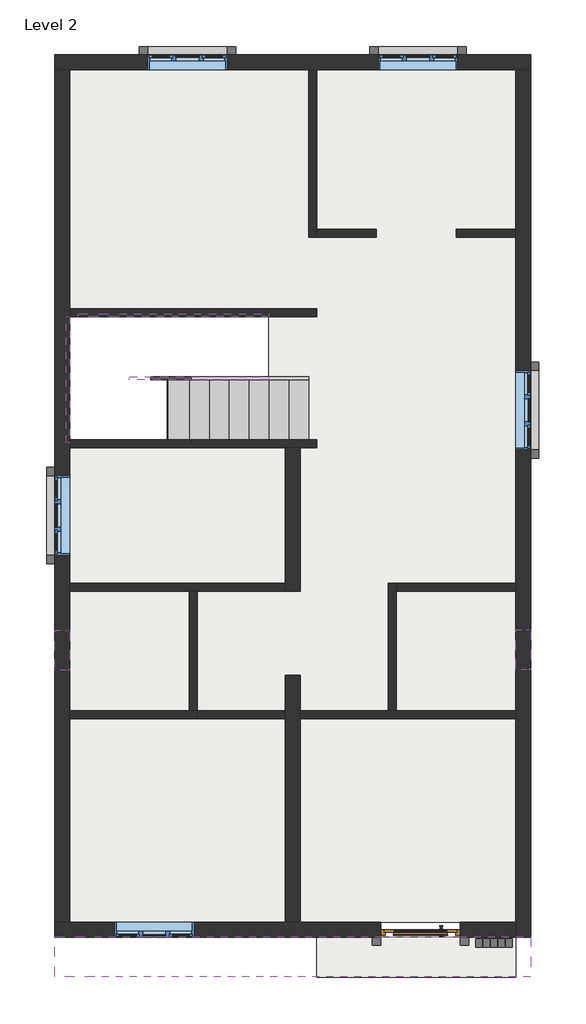
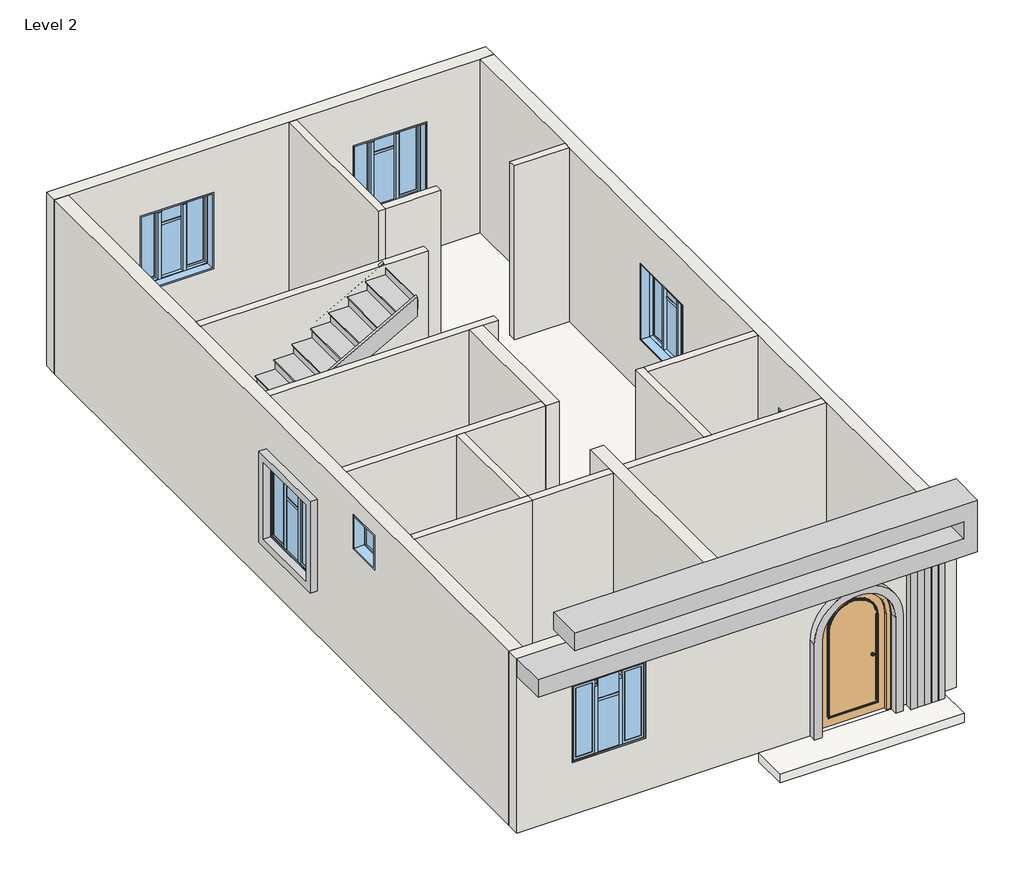
# One storey, incomplete: 18 walls, 7 proxies, 7 windows, 5 members, 4 slabs, 1 door, 1 stair flight.
"""IFC4 building model written with IfcOpenShell, lengths in millimetres."""

from ifc_helpers import new_model, si_unit, frame, origin, place, context, project, spatial, polyline, circle_curve, outline, extrude, faceted_brep, transform, mapped, element, save
from ifc_brep_helpers import plane_surface, revolved_surface, advanced_brep
from components import generic_models_13_generic_models_13_77cabad3, generic_models_14_generic_models_14_97bd1c4e, generic_models_20_generic_models_18_c69d9d0b, generic_models_3_generic_models_3_7bb868d1, generic_models_4_generic_models_4_8dd9e423, generic_models_5_generic_models_5_fe75d143, door_arched_single_french_glass_wood_exterior_1219_x_2134mm_7a906126, stair_flight_03b7873a, window_80340324, window_casement_triple_middle_transom_windows_4_x4_273a115f

model = new_model("IFC4")

# Units and contexts
model_context = context("Model", 3, world=origin())
ifc_project = project(units=[si_unit("LENGTHUNIT", "METRE", prefix="MILLI")], contexts=[model_context])

# Site, building, storey
site = spatial("IfcSite", under=ifc_project)
building = spatial("IfcBuilding", under=site)
storey = spatial("IfcBuildingStorey", under=building, Name="Level 2", Elevation=3352.8)

# Proxies
placement = place(None, origin())
generic_models_13_generic_models_13_shape = generic_models_13_generic_models_13_77cabad3(model_context)
element("IfcBuildingElementProxy", 1, Name="Generic Models 13 : Generic Models 13", ObjectType="Generic Models 13 : Generic Models 13", at=placement, inside=storey, context=model_context, shape_type="MappedRepresentation", body=[
    mapped(generic_models_13_generic_models_13_shape, transform((0.0, 0.0, 0.0), x_axis=(1.0, 0.0, 0.0), y_axis=(0.0, 1.0, 0.0), z_axis=(0.0, 0.0, 1.0))),
])
generic_models_14_generic_models_14_shape = generic_models_14_generic_models_14_97bd1c4e(model_context)
element("IfcBuildingElementProxy", 2, Name="Generic Models 14 : Generic Models 14", ObjectType="Generic Models 14 : Generic Models 14", at=placement, inside=storey, context=model_context, shape_type="MappedRepresentation", body=[
    mapped(generic_models_14_generic_models_14_shape, transform((0.0, 0.0, 0.0), x_axis=(1.0, 0.0, 0.0), y_axis=(0.0, 1.0, 0.0), z_axis=(0.0, 0.0, 1.0))),
])
element("IfcBuildingElementProxy", 3, Name="Generic Models 15 : Generic Models 14", ObjectType="Generic Models 15 : Generic Models 14", at=placement, inside=storey, context=model_context, shape_type="MappedRepresentation", body=[
    mapped(generic_models_14_generic_models_14_shape, transform((-3531.39375, 0.0, 0.0), x_axis=(1.0, 0.0, 0.0), y_axis=(0.0, 1.0, 0.0), z_axis=(0.0, 0.0, 1.0))),
])
generic_models_20_generic_models_18_shape = generic_models_20_generic_models_18_c69d9d0b(model_context)
element("IfcBuildingElementProxy", 4, Name="Generic Models 20 : Generic Models 18", ObjectType="Generic Models 20 : Generic Models 18", at=placement, inside=storey, context=model_context, shape_type="MappedRepresentation", body=[
    mapped(generic_models_20_generic_models_18_shape, transform((0.0, -4883.15, 3041.65), x_axis=(1.0, 0.0, 0.0), y_axis=(0.0, 1.0, 0.0), z_axis=(0.0, 0.0, 1.0))),
])
generic_models_3_generic_models_3_shape = generic_models_3_generic_models_3_7bb868d1(model_context)
element("IfcBuildingElementProxy", 5, Name="Generic Models 3 : Generic Models 3", ObjectType="Generic Models 3 : Generic Models 3", at=placement, inside=storey, context=model_context, shape_type="MappedRepresentation", body=[
    mapped(generic_models_3_generic_models_3_shape, transform((0.0, 0.0, 0.0), x_axis=(1.0, 0.0, 0.0), y_axis=(0.0, 1.0, 0.0), z_axis=(0.0, 0.0, 1.0))),
])
generic_models_4_generic_models_4_shape = generic_models_4_generic_models_4_8dd9e423(model_context)
element("IfcBuildingElementProxy", 6, Name="Generic Models 4 : Generic Models 4", ObjectType="Generic Models 4 : Generic Models 4", at=placement, inside=storey, context=model_context, shape_type="MappedRepresentation", body=[
    mapped(generic_models_4_generic_models_4_shape, transform((0.0, 0.0, 0.0), x_axis=(1.0, 0.0, 0.0), y_axis=(0.0, 1.0, 0.0), z_axis=(0.0, 0.0, 1.0))),
])
generic_models_5_generic_models_5_shape = generic_models_5_generic_models_5_fe75d143(model_context)
element("IfcBuildingElementProxy", 7, Name="Generic Models 5 : Generic Models 5", ObjectType="Generic Models 5 : Generic Models 5", at=placement, inside=storey, context=model_context, shape_type="MappedRepresentation", body=[
    mapped(generic_models_5_generic_models_5_shape, transform((0.0, 0.0, 0.0), x_axis=(1.0, 0.0, 0.0), y_axis=(0.0, 1.0, 0.0), z_axis=(0.0, 0.0, 1.0))),
])

# Door
door_arched_single_french_glass_wood_exterior_1219_x_2134mm_shape = door_arched_single_french_glass_wood_exterior_1219_x_2134mm_7a906126(model_context)
element("IfcDoor", 8, ObjectType="Door_Arched_Single_French_Glass_Wood_Exterior : 1219 x 2134mm", at=placement, inside=storey, context=model_context, shape_type="MappedRepresentation", body=[
    mapped(door_arched_single_french_glass_wood_exterior_1219_x_2134mm_shape, transform((-4097.4482439, -5608.2827462, 3352.8), x_axis=(-1.0, 0.0, 0.0), y_axis=(0.0, -1.0, 0.0), z_axis=(0.0, 0.0, 1.0))),
])

# Members
element("IfcMember", 9, ObjectType="Stringer - 2\" Width", at=placement, inside=storey, context=model_context, shape_type="SweptSolid", body=[
    extrude(outline(polyline([(3352.8, -5811.9482439), (3560.3983948, -5811.9482439), (5122.3333333, -8623.4311333), (5122.3333333, -9251.0527467), (3352.8, -6065.8927467), (3352.8, -5811.9482439)])), frame((0.0, 1846.6172538, 0.0), z_axis=(0.0, 1.0, 0.0), x_axis=(0.0, 0.0, 1.0)), (0.0, 0.0, 1.0), 50.8),
])
element("IfcMember", 10, ObjectType="Stringer - 2\" Width", at=placement, inside=storey, context=model_context, shape_type="SweptSolid", body=[
    extrude(outline(polyline([(-9471.1357439, 1846.6172538), (-9521.9357439, 1846.6172538), (-9521.9357439, 3777.0172538), (-9471.1357439, 3777.0172538), (-9471.1357439, 1846.6172538)])), frame((0.0, 0.0, 4817.5333333), z_axis=(0.0, 0.0, 1.0), x_axis=(1.0, 0.0, 0.0)), (0.0, 0.0, 1.0), 304.8),
])
element("IfcMember", 11, ObjectType="Stringer - 2\" Width", at=placement, inside=storey, context=model_context, shape_type="SweptSolid", body=[
    extrude(outline(polyline([(4817.5333333, -8712.6837411), (6090.3863873, -6421.5482439), (6439.0650614, -6421.5482439), (4817.5333333, -9340.3053545), (4817.5333333, -8712.6837411)])), frame((0.0, 3777.0172538, 0.0), z_axis=(0.0, 1.0, 0.0), x_axis=(0.0, 0.0, 1.0)), (0.0, 0.0, 1.0), 50.8),
])
element("IfcMember", 12, ObjectType="Stringer - 2\" Width", at=placement, inside=storey, context=model_context, shape_type="SweptSolid", body=[
    extrude(outline(polyline([(3352.8, -5811.9482439), (3560.3983948, -5811.9482439), (5056.1761726, -8504.3482439), (4707.4974984, -8504.3482439), (3352.8, -6065.8927467), (3352.8, -5811.9482439)])), frame((0.0, 2811.8172538, 0.0), z_axis=(0.0, 1.0, 0.0), x_axis=(0.0, 0.0, 1.0)), (0.0, 0.0, 1.0), 50.8),
])
element("IfcMember", 13, ObjectType="Stringer - 2\" Width", at=placement, inside=storey, context=model_context, shape_type="SweptSolid", body=[
    extrude(outline(polyline([(5253.7317281, -8555.1482439), (4905.053054, -8555.1482439), (6090.3863873, -6421.5482439), (6439.0650614, -6421.5482439), (5253.7317281, -8555.1482439)])), frame((0.0, 2811.8172538, 0.0), z_axis=(0.0, 1.0, 0.0), x_axis=(0.0, 0.0, 1.0)), (0.0, 0.0, 1.0), 50.8),
])

# Slabs
element("IfcSlab", 14, ObjectType="6\" flooring bathroom second lvl", at=placement, inside=storey, context=model_context, shape_type="SweptSolid", body=[
    extrude(outline(polyline([(-7640.7482439, -426.6827462), (-7640.7482439, -2255.4827462), (-9471.1357439, -2255.4827462), (-9471.1357439, -426.6827462), (-7640.7482439, -426.6827462)])), frame((0.0, 0.0, 3200.4), z_axis=(0.0, 0.0, 1.0), x_axis=(1.0, 0.0, 0.0)), (0.0, 0.0, 1.0), 152.4),
    extrude(outline(polyline([(-2636.9482439, -426.6827462), (-2636.9482439, -2255.4827462), (-4465.7482439, -2255.4827462), (-4465.7482439, -426.6827462), (-2636.9482439, -426.6827462)])), frame((0.0, 0.0, 3200.4), z_axis=(0.0, 0.0, 1.0), x_axis=(1.0, 0.0, 0.0)), (0.0, 0.0, 1.0), 152.4),
])
element("IfcSlab", 15, ObjectType="6\" flooring bathroom second lvl", at=placement, inside=storey, context=model_context, shape_type="SweptSolid", body=[
    extrude(outline(polyline([(-2635.3607439, -5722.5827462), (-2635.3607439, -6341.8842658), (-5683.3607439, -6341.8842658), (-5683.3607439, -5722.5827462), (-2635.3607439, -5722.5827462)])), frame((0.0, 0.0, 3200.4), z_axis=(0.0, 0.0, 1.0), x_axis=(1.0, 0.0, 0.0)), (0.0, 0.0, 1.0), 152.4),
])
element("IfcSlab", 16, ObjectType="flooring 6\"", at=placement, inside=storey, context=model_context, shape_type="SweptSolid", body=[
    extrude(outline(polyline([(-9471.1357439, 3904.0172538), (-9471.1357439, 7563.2047538), (-5811.9482439, 7563.2047538), (-5811.9482439, 4996.2172538), (-4770.5482439, 4996.2172538), (-4770.5482439, 5123.2172538), (-5684.9482439, 5123.2172538), (-5684.9482439, 7563.2047538), (-2636.9482439, 7563.2047538), (-2636.9482439, 5123.2172538), (-3551.3482439, 5123.2172538), (-3551.3482439, 4996.2172538), (-2636.9482439, 4996.2172538), (-2636.9482439, -299.6827462), (-4592.7482439, -299.6827462), (-4592.7482439, -2255.4827462), (-5936.4082439, -2255.4827462), (-5936.4082439, -1709.3827462), (-6165.0082439, -1709.3827462), (-6165.0082439, -2255.4827462), (-6170.0882439, -2255.4827462), (-7513.7482439, -2255.4827462), (-7513.7482439, -426.6827462), (-5936.4082439, -426.6827462), (-5936.4082439, 1770.4172538), (-5684.9482439, 1770.4172538), (-5684.9482439, 1897.4172538), (-5811.9482439, 1897.4172538), (-5811.9482439, 2862.6172538), (-6421.5482439, 2862.6172538), (-6421.5482439, 3777.0172538), (-5684.9482439, 3777.0172538), (-5684.9482439, 3904.0172538), (-9471.1357439, 3904.0172538)])), frame((0.0, 0.0, 3200.4), z_axis=(0.0, 0.0, 1.0), x_axis=(1.0, 0.0, 0.0)), (0.0, 0.0, 1.0), 152.4),
])
element("IfcSlab", 17, ObjectType="flooring 6\"", at=placement, inside=storey, context=model_context, shape_type="SweptSolid", body=[
    extrude(outline(polyline([(-6165.0082439, 1770.4172538), (-6165.0082439, -299.6827462), (-9471.1357439, -299.6827462), (-9471.1357439, 1770.4172538), (-6165.0082439, 1770.4172538)])), frame((0.0, 0.0, 3327.4), z_axis=(0.0, 0.0, 1.0), x_axis=(1.0, 0.0, 0.0)), (0.0, 0.0, 1.0), 152.4),
    extrude(outline(polyline([(-6170.0882439, -5493.9827462), (-9471.1357439, -5493.9827462), (-9471.1357439, -2382.4827462), (-6170.0882439, -2382.4827462), (-6170.0882439, -5493.9827462)])), frame((0.0, 0.0, 3327.4), z_axis=(0.0, 0.0, 1.0), x_axis=(1.0, 0.0, 0.0)), (0.0, 0.0, 1.0), 152.4),
    extrude(outline(polyline([(-2636.9482439, -2382.4827462), (-2636.9482439, -5493.9827462), (-5936.4082439, -5493.9827462), (-5936.4082439, -2382.4827462), (-2636.9482439, -2382.4827462)])), frame((0.0, 0.0, 3327.4), z_axis=(0.0, 0.0, 1.0), x_axis=(1.0, 0.0, 0.0)), (0.0, 0.0, 1.0), 152.4),
])

# Stair flight
stair_flight_shape = stair_flight_03b7873a(model_context)
element("IfcStairFlight", 18, ObjectType="2\" Tread 1\" Nosing 1/4\" Riser", at=placement, inside=storey, context=model_context, shape_type="MappedRepresentation", body=[
    mapped(stair_flight_shape, transform((0.0, 0.0, 0.0), x_axis=(1.0, 0.0, 0.0), y_axis=(0.0, 1.0, 0.0), z_axis=(0.0, 0.0, 1.0))),
])

# Walls
element("IfcWall", 19, ObjectType="INNER WALL 5\"", at=placement, inside=storey, context=model_context, shape_type="SweptSolid", body=[
    extrude(outline(polyline([(-5684.9482439, 3777.0172538), (-9471.1357439, 3777.0172538), (-9471.1357439, 3904.0172538), (-5684.9482439, 3904.0172538), (-5684.9482439, 3777.0172538)])), frame((0.0, 0.0, 3352.8), z_axis=(0.0, 0.0, 1.0), x_axis=(1.0, 0.0, 0.0)), (0.0, 0.0, 1.0), 3048.0),
])
element("IfcWall", 20, ObjectType="INNER WALL 5\"", at=placement, inside=storey, context=model_context, shape_type="Brep", body=[
    faceted_brep([(-9471.1357439, 1770.4172538, 3352.8), (-6165.0082439, 1770.4172538, 3352.8), (-5936.4082439, 1770.4172538, 3352.8), (-5684.9482439, 1770.4172538, 3352.8), (-5684.9482439, 1770.4172538, 6400.8), (-5936.4082439, 1770.4172538, 6400.8), (-6165.0082439, 1770.4172538, 6400.8), (-9471.1357439, 1770.4172538, 6400.8), (-9471.1357439, 1897.4172538, 3352.8), (-9471.1357439, 1897.4172538, 6400.8), (-5684.9482439, 1897.4172538, 6400.8), (-5684.9482439, 1897.4172538, 3352.8)], [[[0, 1, 2, 3, 4, 5, 6, 7]], [[8, 9, 10, 11]], [[3, 2, 1, 0, 8, 11]], [[4, 3, 11, 10]], [[7, 6, 5, 4, 10, 9]], [[0, 7, 9, 8]]]),
])
element("IfcWall", 21, ObjectType="INNER WALL 5\"", at=placement, inside=storey, context=model_context, shape_type="Brep", body=[
    faceted_brep([(-9471.1357439, -426.6827462, 3352.8), (-7640.7482439, -426.6827462, 3352.8), (-7513.7482439, -426.6827462, 3352.8), (-6165.0082439, -426.6827462, 3352.8), (-6165.0082439, -426.6827462, 6400.8), (-7513.7482439, -426.6827462, 6400.8), (-7640.7482439, -426.6827462, 6400.8), (-9471.1357439, -426.6827462, 6400.8), (-9471.1357439, -299.6827462, 3352.8), (-9471.1357439, -299.6827462, 6400.8), (-6165.0082439, -299.6827462, 6400.8), (-6165.0082439, -299.6827462, 3352.8)], [[[0, 1, 2, 3, 4, 5, 6, 7]], [[8, 9, 10, 11]], [[3, 2, 1, 0, 8, 11]], [[7, 6, 5, 4, 10, 9]], [[4, 3, 11, 10]], [[0, 7, 9, 8]]]),
])
element("IfcWall", 22, ObjectType="INNER WALL 5\"", at=placement, inside=storey, context=model_context, shape_type="Brep", body=[
    faceted_brep([(-9469.5482439, -2382.4827462, 3352.8), (-7513.7482439, -2382.4827462, 3352.8), (-7513.7482439, -2382.4827462, 6400.8), (-9469.5482439, -2382.4827462, 6400.8), (-9469.5482439, -2255.4827462, 3352.8), (-9469.5482439, -2255.4827462, 6400.8), (-7640.7482439, -2255.4827462, 6400.8), (-7513.7482439, -2255.4827462, 6400.8), (-7513.7482439, -2255.4827462, 3352.8), (-7640.7482439, -2255.4827462, 3352.8)], [[[0, 1, 2, 3]], [[4, 5, 6, 7, 8, 9]], [[1, 0, 4, 9, 8]], [[3, 2, 7, 6, 5]], [[0, 3, 5, 4]], [[2, 1, 8, 7]]]),
])
element("IfcWall", 23, ObjectType="INNER WALL 5\"", at=placement, inside=storey, context=model_context, shape_type="SweptSolid", body=[
    extrude(outline(polyline([(-7513.7482439, -426.6827462), (-7513.7482439, -2255.4827462), (-7640.7482439, -2255.4827462), (-7640.7482439, -426.6827462), (-7513.7482439, -426.6827462)])), frame((0.0, 0.0, 3352.8), z_axis=(0.0, 0.0, 1.0), x_axis=(1.0, 0.0, 0.0)), (0.0, 0.0, 1.0), 3048.0),
])
element("IfcWall", 24, ObjectType="INNER WALL 5\"", at=placement, inside=storey, context=model_context, shape_type="SweptSolid", body=[
    extrude(outline(polyline([(-7513.7482439, -2255.4827462), (-6170.0882439, -2255.4827462), (-6170.0882439, -2382.4827462), (-7513.7482439, -2382.4827462), (-7513.7482439, -2255.4827462)])), frame((0.0, 0.0, 3352.8), z_axis=(0.0, 0.0, 1.0), x_axis=(1.0, 0.0, 0.0)), (0.0, 0.0, 1.0), 3048.0),
])
element("IfcWall", 25, ObjectType="INNER WALL 5\"", at=placement, inside=storey, context=model_context, shape_type="Brep", body=[
    faceted_brep([(-5936.4082439, -2382.4827462, 3352.8), (-2636.9482439, -2382.4827462, 3352.8), (-2636.9482439, -2382.4827462, 6400.8), (-5936.4082439, -2382.4827462, 6400.8), (-5936.4082439, -2255.4827462, 3352.8), (-5936.4082439, -2255.4827462, 6400.8), (-4592.7482439, -2255.4827462, 6400.8), (-4465.7482439, -2255.4827462, 6400.8), (-2636.9482439, -2255.4827462, 6400.8), (-2636.9482439, -2255.4827462, 3352.8), (-4465.7482439, -2255.4827462, 3352.8), (-4592.7482439, -2255.4827462, 3352.8)], [[[0, 1, 2, 3]], [[4, 5, 6, 7, 8, 9, 10, 11]], [[1, 0, 4, 11, 10, 9]], [[3, 2, 8, 7, 6, 5]], [[0, 3, 5, 4]], [[2, 1, 9, 8]]]),
])
element("IfcWall", 26, ObjectType="INNER WALL 5\"", at=placement, inside=storey, context=model_context, shape_type="Brep", body=[
    faceted_brep([(-4465.7482439, -2255.4827462, 3352.8), (-4465.7482439, -426.6827462, 3352.8), (-4465.7482439, -299.6827462, 3352.8), (-4465.7482439, -299.6827462, 6400.8), (-4465.7482439, -426.6827462, 6400.8), (-4465.7482439, -2255.4827462, 6400.8), (-4592.7482439, -2255.4827462, 3352.8), (-4592.7482439, -2255.4827462, 6400.8), (-4592.7482439, -299.6827462, 6400.8), (-4592.7482439, -299.6827462, 3352.8)], [[[0, 1, 2, 3, 4, 5]], [[6, 7, 8, 9]], [[2, 1, 0, 6, 9]], [[5, 4, 3, 8, 7]], [[0, 5, 7, 6]], [[3, 2, 9, 8]]]),
])
element("IfcWall", 27, ObjectType="INNER WALL 5\"", at=placement, inside=storey, context=model_context, shape_type="SweptSolid", body=[
    extrude(outline(polyline([(-2636.9482439, -426.6827462), (-4465.7482439, -426.6827462), (-4465.7482439, -299.6827462), (-2636.9482439, -299.6827462), (-2636.9482439, -426.6827462)])), frame((0.0, 0.0, 3352.8), z_axis=(0.0, 0.0, 1.0), x_axis=(1.0, 0.0, 0.0)), (0.0, 0.0, 1.0), 3048.0),
])
element("IfcWall", 28, ObjectType="INNER WALL 5\"", at=placement, inside=storey, context=model_context, shape_type="Brep", body=[
    faceted_brep([(-5811.9482439, 7563.2047538, 3352.8), (-5811.9482439, 4996.2172538, 3352.8), (-5811.9482439, 4996.2172538, 6400.8), (-5811.9482439, 7563.2047538, 6400.8), (-5684.9482439, 7563.2047538, 3352.8), (-5684.9482439, 7563.2047538, 6400.8), (-5684.9482439, 5123.2172538, 6400.8), (-5684.9482439, 4996.2172538, 6400.8), (-5684.9482439, 4996.2172538, 3352.8), (-5684.9482439, 5123.2172538, 3352.8)], [[[0, 1, 2, 3]], [[4, 5, 6, 7, 8, 9]], [[1, 0, 4, 9, 8]], [[3, 2, 7, 6, 5]], [[0, 3, 5, 4]], [[2, 1, 8, 7]]]),
])
element("IfcWall", 29, ObjectType="INNER WALL 5\"", at=placement, inside=storey, context=model_context, shape_type="SweptSolid", body=[
    extrude(outline(polyline([(-4770.5482439, 4996.2172538), (-5684.9482439, 4996.2172538), (-5684.9482439, 5123.2172538), (-4770.5482439, 5123.2172538), (-4770.5482439, 4996.2172538)])), frame((0.0, 0.0, 3352.8), z_axis=(0.0, 0.0, 1.0), x_axis=(1.0, 0.0, 0.0)), (0.0, 0.0, 1.0), 3048.0),
])
element("IfcWall", 30, ObjectType="INNER WALL 5\"", at=placement, inside=storey, context=model_context, shape_type="SweptSolid", body=[
    extrude(outline(polyline([(-2636.9482439, 4996.2172538), (-3551.3482439, 4996.2172538), (-3551.3482439, 5123.2172538), (-2636.9482439, 5123.2172538), (-2636.9482439, 4996.2172538)])), frame((0.0, 0.0, 3352.8), z_axis=(0.0, 0.0, 1.0), x_axis=(1.0, 0.0, 0.0)), (0.0, 0.0, 1.0), 3048.0),
])
element("IfcWall", 31, ObjectType="WALL 9\"", at=placement, inside=storey, context=model_context, shape_type="Brep", body=[
    faceted_brep([(-9699.7357439, 7563.2047538, 3352.8), (-9471.1357439, 7563.2047538, 3352.8), (-5811.9482439, 7563.2047538, 3352.8), (-5684.9482439, 7563.2047538, 3352.8), (-2636.9482439, 7563.2047538, 3352.8), (-2408.3482439, 7563.2047538, 3352.8), (-2408.3482439, 7563.2047538, 6400.8), (-2636.9482439, 7563.2047538, 6400.8), (-5684.9482439, 7563.2047538, 6400.8), (-5811.9482439, 7563.2047538, 6400.8), (-9471.1357439, 7563.2047538, 6400.8), (-9699.7357439, 7563.2047538, 6400.8), (-3525.9482439, 7563.2047538, 5613.4), (-3525.9482439, 7563.2047538, 4267.2), (-4745.1482439, 7563.2047538, 4267.2), (-4745.1482439, 7563.2047538, 5613.4), (-7057.3419939, 7563.2047538, 5613.4), (-7057.3419939, 7563.2047538, 4267.2), (-8276.5419939, 7563.2047538, 4267.2), (-8276.5419939, 7563.2047538, 5613.4), (-9699.7357439, 7791.8047538, 3352.8), (-9699.7357439, 7791.8047538, 6400.8), (-2408.3482439, 7791.8047538, 6400.8), (-2408.3482439, 7791.8047538, 3352.8), (-3525.9482439, 7791.8047538, 5613.4), (-4745.1482439, 7791.8047538, 5613.4), (-4745.1482439, 7791.8047538, 4267.2), (-3525.9482439, 7791.8047538, 4267.2), (-7057.3419939, 7791.8047538, 5613.4), (-8276.5419939, 7791.8047538, 5613.4), (-8276.5419939, 7791.8047538, 4267.2), (-7057.3419939, 7791.8047538, 4267.2)], [[[0, 1, 2, 3, 4, 5, 6, 7, 8, 9, 10, 11], [12, 13, 14, 15], [16, 17, 18, 19]], [[20, 21, 22, 23], [24, 25, 26, 27], [28, 29, 30, 31]], [[5, 4, 3, 2, 1, 0, 20, 23]], [[11, 10, 9, 8, 7, 6, 22, 21]], [[6, 5, 23, 22]], [[0, 11, 21, 20]], [[13, 12, 24, 27]], [[14, 13, 27, 26]], [[15, 14, 26, 25]], [[12, 15, 25, 24]], [[17, 16, 28, 31]], [[18, 17, 31, 30]], [[19, 18, 30, 29]], [[16, 19, 29, 28]]]),
])
element("IfcWall", 32, ObjectType="WALL 9\"", at=placement, inside=storey, context=model_context, shape_type="Brep", body=[
    faceted_brep([(-2636.9482439, 7563.2047538, 3352.8), (-2636.9482439, 5123.2172538, 3352.8), (-2636.9482439, 4996.2172538, 3352.8), (-2636.9482439, -299.6827462, 3352.8), (-2636.9482439, -426.6827462, 3352.8), (-2636.9482439, -2255.4827462, 3352.8), (-2636.9482439, -2382.4827462, 3352.8), (-2636.9482439, -5493.9827462, 3352.8), (-2636.9482439, -5722.5827462, 3352.8), (-2636.9482439, -5722.5827462, 6400.8), (-2636.9482439, -5493.9827462, 6400.8), (-2636.9482439, -2382.4827462, 6400.8), (-2636.9482439, -2255.4827462, 6400.8), (-2636.9482439, -426.6827462, 6400.8), (-2636.9482439, -299.6827462, 6400.8), (-2636.9482439, 4996.2172538, 6400.8), (-2636.9482439, 5123.2172538, 6400.8), (-2636.9482439, 7563.2047538, 6400.8), (-2636.9482439, 1738.6672538, 5613.4), (-2636.9482439, 1738.6672538, 4267.2), (-2636.9482439, 2957.8672538, 4267.2), (-2636.9482439, 2957.8672538, 5613.4), (-2636.9482439, -1626.8327462, 5486.4), (-2636.9482439, -1626.8327462, 4876.8), (-2636.9482439, -1017.2327462, 4876.8), (-2636.9482439, -1017.2327462, 5486.4), (-2408.3482439, 7563.2047538, 3352.8), (-2408.3482439, 7563.2047538, 6400.8), (-2408.3482439, -5722.5827462, 6400.8), (-2408.3482439, -5722.5827462, 3352.8), (-2408.3482439, 1738.6672538, 5613.4), (-2408.3482439, 2957.8672538, 5613.4), (-2408.3482439, 2957.8672538, 4267.2), (-2408.3482439, 1738.6672538, 4267.2), (-2408.3482439, -1626.8327462, 5486.4), (-2408.3482439, -1017.2327462, 5486.4), (-2408.3482439, -1017.2327462, 4876.8), (-2408.3482439, -1626.8327462, 4876.8)], [[[0, 1, 2, 3, 4, 5, 6, 7, 8, 9, 10, 11, 12, 13, 14, 15, 16, 17], [18, 19, 20, 21], [22, 23, 24, 25]], [[26, 27, 28, 29], [30, 31, 32, 33], [34, 35, 36, 37]], [[8, 7, 6, 5, 4, 3, 2, 1, 0, 26, 29]], [[17, 16, 15, 14, 13, 12, 11, 10, 9, 28, 27]], [[0, 17, 27, 26]], [[9, 8, 29, 28]], [[19, 18, 30, 33]], [[20, 19, 33, 32]], [[21, 20, 32, 31]], [[18, 21, 31, 30]], [[23, 22, 34, 37]], [[24, 23, 37, 36]], [[25, 24, 36, 35]], [[22, 25, 35, 34]]]),
])
element("IfcWall", 33, ObjectType="WALL 9\"", at=placement, inside=storey, context=model_context, shape_type="AdvancedBrep", body=[
    advanced_brep(
    [(-4707.0482439, -5493.9827462, 5031.4), (-4707.0482439, -5493.9827462, 3352.8), (-5936.4082439, -5493.9827462, 3352.8), (-6165.0082439, -5493.9827462, 3352.8), (-9471.1357439, -5493.9827462, 3352.8), (-9699.7357439, -5493.9827462, 3352.8), (-9699.7357439, -5493.9827462, 6400.8), (-9471.1357439, -5493.9827462, 6400.8), (-6165.0082439, -5493.9827462, 6400.8), (-5936.4082439, -5493.9827462, 6400.8), (-2636.9482439, -5493.9827462, 6400.8), (-2636.9482439, -5493.9827462, 3352.8), (-3487.8482439, -5493.9827462, 3352.8), (-3487.8482439, -5493.9827462, 5031.4), (-8783.2719939, -5493.9827462, 5613.4), (-8783.2719939, -5493.9827462, 4267.2), (-7564.0719939, -5493.9827462, 4267.2), (-7564.0719939, -5493.9827462, 5613.4), (-9699.7357439, -5722.5827462, 3352.8), (-4707.0482439, -5722.5827462, 3352.8), (-4707.0482439, -5722.5827462, 5031.4), (-3487.8482439, -5722.5827462, 5031.4), (-3487.8482439, -5722.5827462, 3352.8), (-2636.9482439, -5722.5827462, 3352.8), (-2636.9482439, -5722.5827462, 6400.8), (-9699.7357439, -5722.5827462, 6400.8), (-8783.2719939, -5722.5827462, 5613.4), (-7564.0719939, -5722.5827462, 5613.4), (-7564.0719939, -5722.5827462, 4267.2), (-8783.2719939, -5722.5827462, 4267.2)],
    [
        (0, 1),
        (1, 2),
        (2, 3),
        (3, 4),
        (4, 5),
        (5, 6),
        (6, 7),
        (7, 8),
        (8, 9),
        (9, 10),
        (10, 11),
        (11, 12),
        (12, 13),
        (13, 0, circle_curve(frame((-4097.4482439, -5493.9827462, 5031.4), z_axis=(0.0, -1.0, 0.0), x_axis=(-1.0, 0.0, 0.0)), 609.6)),
        (14, 15),
        (15, 16),
        (16, 17),
        (17, 14),
        (18, 19),
        (19, 20),
        (20, 21, circle_curve(frame((-4097.4482439, -5722.5827462, 5031.4), z_axis=(0.0, 1.0, 0.0), x_axis=(-1.0, 0.0, 0.0)), 609.6)),
        (21, 22),
        (22, 23),
        (23, 24),
        (24, 25),
        (25, 18),
        (26, 27),
        (27, 28),
        (28, 29),
        (29, 26),
        (11, 23),
        (22, 12),
        (1, 19),
        (18, 5),
        (6, 25),
        (24, 10),
        (14, 26),
        (29, 15),
        (28, 16),
        (27, 17),
        (20, 0),
        (13, 21),
    ],
    [
        plane_surface(frame((-2408.3482439, -5493.9827462, 3352.8), z_axis=(0.0, 1.0, 0.0), x_axis=(-1.0, 0.0, 0.0))),
        plane_surface(frame((-2408.3482439, -5722.5827462, 3352.8), z_axis=(0.0, -1.0, 0.0), x_axis=(1.0, 0.0, 0.0))),
        plane_surface(frame((-2522.6482439, -5493.9827462, 3352.8), z_axis=(0.0, 0.0, -1.0), x_axis=(0.0, -1.0, 0.0))),
        plane_surface(frame((-9585.4357439, -5493.9827462, 6400.8), z_axis=(0.0, 0.0, 1.0), x_axis=(0.0, -1.0, 0.0))),
        plane_surface(frame((-2636.9482439, 7551.109711, 3352.8), z_axis=(1.0, 0.0, 0.0), x_axis=(0.0, -1.0, 0.0))),
        plane_surface(frame((-9699.7357439, -5722.5827462, 3352.8), z_axis=(-1.0, 0.0, 0.0), x_axis=(0.0, -1.0, 0.0))),
        plane_surface(frame((-8783.2719939, -5493.9827462, 5613.4), z_axis=(1.0, 0.0, 0.0), x_axis=(0.0, -1.0, 0.0))),
        plane_surface(frame((-8783.2719939, -5493.9827462, 4267.2), z_axis=(0.0, 0.0, 1.0), x_axis=(0.0, -1.0, 0.0))),
        plane_surface(frame((-7564.0719939, -5493.9827462, 4267.2), z_axis=(-1.0, 0.0, 0.0), x_axis=(0.0, -1.0, 0.0))),
        plane_surface(frame((-7564.0719939, -5493.9827462, 5613.4), z_axis=(0.0, 0.0, -1.0), x_axis=(0.0, -1.0, 0.0))),
        revolved_surface(polyline([(-4707.048243900001, -5493.9827462, 5031.4), (-4707.048243900001, -5722.5827462, 5031.4)]), (-4097.4482439, -5493.9827462, 5031.4), (0.0, 1.0, 0.0)),
        plane_surface(frame((-3487.8482439, -5722.5827462, 5031.4), z_axis=(-1.0, 0.0, 0.0), x_axis=(0.0, 1.0, 0.0))),
        plane_surface(frame((-4707.0482439, -5722.5827462, 3352.8), z_axis=(1.0, 0.0, 0.0), x_axis=(0.0, 1.0, 0.0))),
    ],
    [
        (0, [[1, 2, 3, 4, 5, 6, 7, 8, 9, 10, 11, 12, 13, 14], [15, 16, 17, 18]]),
        (1, [[19, 20, 21, 22, 23, 24, 25, 26], [27, 28, 29, 30]]),
        (2, [[-12, 31, -23, 32]]),
        (2, [[-5, -4, -3, -2, 33, -19, 34]]),
        (3, [[-10, -9, -8, -7, 35, -25, 36]]),
        (4, [[-11, -36, -24, -31]]),
        (5, [[-6, -34, -26, -35]]),
        (6, [[-15, 37, -30, 38]]),
        (7, [[-16, -38, -29, 39]]),
        (8, [[-17, -39, -28, 40]]),
        (9, [[-18, -40, -27, -37]]),
        (10, [[-21, 41, -14, 42]]),
        (11, [[-22, -42, -13, -32]]),
        (12, [[-20, -33, -1, -41]]),
    ],
),
])
element("IfcWall", 34, ObjectType="WALL 9\"", at=placement, inside=storey, context=model_context, shape_type="Brep", body=[
    faceted_brep([(-9471.1357439, -5493.9827462, 3352.8), (-9471.1357439, -426.6827462, 3352.8), (-9471.1357439, -299.6827462, 3352.8), (-9471.1357439, 1770.4172538, 3352.8), (-9471.1357439, 1897.4172538, 3352.8), (-9471.1357439, 3777.0172538, 3352.8), (-9471.1357439, 3904.0172538, 3352.8), (-9471.1357439, 7563.2047538, 3352.8), (-9471.1357439, 7563.2047538, 6400.8), (-9471.1357439, 3904.0172538, 6400.8), (-9471.1357439, 3777.0172538, 6400.8), (-9471.1357439, 1897.4172538, 6400.8), (-9471.1357439, 1770.4172538, 6400.8), (-9471.1357439, -299.6827462, 6400.8), (-9471.1357439, -426.6827462, 6400.8), (-9471.1357439, -5493.9827462, 6400.8), (-9471.1357439, 1344.9672538, 5613.4), (-9471.1357439, 1344.9672538, 4267.2), (-9471.1357439, 125.7672538, 4267.2), (-9471.1357439, 125.7672538, 5613.4), (-9471.1357439, -1633.1827462, 6096.0), (-9471.1357439, -1023.5827462, 6096.0), (-9471.1357439, -1023.5827462, 5486.4), (-9471.1357439, -1633.1827462, 5486.4), (-9699.7357439, -5493.9827462, 3352.8), (-9699.7357439, -5493.9827462, 6400.8), (-9699.7357439, 7563.2047538, 6400.8), (-9699.7357439, 7563.2047538, 3352.8), (-9699.7357439, 1344.9672538, 5613.4), (-9699.7357439, 125.7672538, 5613.4), (-9699.7357439, 125.7672538, 4267.2), (-9699.7357439, 1344.9672538, 4267.2), (-9699.7357439, -1633.1827462, 6096.0), (-9699.7357439, -1633.1827462, 5486.4), (-9699.7357439, -1023.5827462, 5486.4), (-9699.7357439, -1023.5827462, 6096.0)], [[[0, 1, 2, 3, 4, 5, 6, 7, 8, 9, 10, 11, 12, 13, 14, 15], [16, 17, 18, 19], [20, 21, 22, 23]], [[24, 25, 26, 27], [28, 29, 30, 31], [32, 33, 34, 35]], [[7, 6, 5, 4, 3, 2, 1, 0, 24, 27]], [[15, 14, 13, 12, 11, 10, 9, 8, 26, 25]], [[0, 15, 25, 24]], [[8, 7, 27, 26]], [[17, 16, 28, 31]], [[18, 17, 31, 30]], [[19, 18, 30, 29]], [[16, 19, 29, 28]], [[33, 32, 20, 23]], [[34, 33, 23, 22]], [[35, 34, 22, 21]], [[32, 35, 21, 20]]]),
])
element("IfcWall", 35, ObjectType="WALL 9\"", at=placement, inside=storey, context=model_context, shape_type="Brep", body=[
    faceted_brep([(-5936.4082439, -5493.9827462, 3352.8), (-5936.4082439, -2382.4827462, 3352.8), (-5936.4082439, -2255.4827462, 3352.8), (-5936.4082439, -1709.3827462, 3352.8), (-5936.4082439, -1709.3827462, 6400.8), (-5936.4082439, -2255.4827462, 6400.8), (-5936.4082439, -2382.4827462, 6400.8), (-5936.4082439, -5493.9827462, 6400.8), (-6165.0082439, -5493.9827462, 3352.8), (-6165.0082439, -5493.9827462, 6400.8), (-6165.0082439, -1709.3827462, 6400.8), (-6165.0082439, -1709.3827462, 3352.8)], [[[0, 1, 2, 3, 4, 5, 6, 7]], [[8, 9, 10, 11]], [[3, 2, 1, 0, 8, 11]], [[4, 3, 11, 10]], [[7, 6, 5, 4, 10, 9]], [[0, 7, 9, 8]]]),
])
element("IfcWall", 36, ObjectType="WALL 9\"", at=placement, inside=storey, context=model_context, shape_type="Brep", body=[
    faceted_brep([(-6165.0082439, 1770.4172538, 3352.8), (-6165.0082439, -299.6827462, 3352.8), (-6165.0082439, -426.6827462, 3352.8), (-6165.0082439, -426.6827462, 6400.8), (-6165.0082439, -299.6827462, 6400.8), (-6165.0082439, 1770.4172538, 6400.8), (-5936.4082439, 1770.4172538, 3352.8), (-5936.4082439, 1770.4172538, 6400.8), (-5936.4082439, -426.6827462, 6400.8), (-5936.4082439, -426.6827462, 3352.8)], [[[0, 1, 2, 3, 4, 5]], [[6, 7, 8, 9]], [[2, 1, 0, 6, 9]], [[5, 4, 3, 8, 7]], [[0, 5, 7, 6]], [[3, 2, 9, 8]]]),
])

# Windows
window_shape = window_80340324(model_context)
element("IfcWindow", 37, ObjectType="Fixed : 24\" x 24\"", at=placement, inside=storey, context=model_context, shape_type="MappedRepresentation", body=[
    mapped(window_shape, transform((-9585.4357439, -1366.4827462, 4572.0), x_axis=(0.0, -1.0, 0.0), y_axis=(1.0, 0.0, 0.0), z_axis=(0.0, 0.0, 1.0))),
])
element("IfcWindow", 38, ObjectType="Fixed : 24\" x 24\"", at=placement, inside=storey, context=model_context, shape_type="MappedRepresentation", body=[
    mapped(window_shape, transform((-2522.6482439, -1360.1327462, 3962.4), x_axis=(0.0, -1.0, 0.0), y_axis=(1.0, 0.0, 0.0), z_axis=(0.0, 0.0, 1.0))),
])
window_casement_triple_middle_transom_windows_4_x4_shape = window_casement_triple_middle_transom_windows_4_x4_273a115f(model_context)
element("IfcWindow", 39, ObjectType="Window-Casement-Triple-Middle-Transom : WINDOWS 4'X4'", at=placement, inside=storey, context=model_context, shape_type="MappedRepresentation", body=[
    mapped(window_casement_triple_middle_transom_windows_4_x4_shape, transform((-8173.6719939, -5608.2827462, 3352.8), x_axis=(-1.0, 0.0, 0.0), y_axis=(0.0, -1.0, 0.0), z_axis=(0.0, 0.0, 1.0))),
])
element("IfcWindow", 40, ObjectType="Window-Casement-Triple-Middle-Transom : WINDOWS 4'X4'", at=placement, inside=storey, context=model_context, shape_type="MappedRepresentation", body=[
    mapped(window_casement_triple_middle_transom_windows_4_x4_shape, transform((-2522.6482439, 2348.2672538, 3352.8), x_axis=(0.0, -1.0, 0.0), y_axis=(1.0, 0.0, 0.0), z_axis=(0.0, 0.0, 1.0))),
])
element("IfcWindow", 41, ObjectType="Window-Casement-Triple-Middle-Transom : WINDOWS 4'X4'", at=placement, inside=storey, context=model_context, shape_type="MappedRepresentation", body=[
    mapped(window_casement_triple_middle_transom_windows_4_x4_shape, transform((-4135.5482439, 7677.5047538, 3352.8), x_axis=(1.0, 0.0, 0.0), y_axis=(0.0, 1.0, 0.0), z_axis=(0.0, 0.0, 1.0))),
])
element("IfcWindow", 42, ObjectType="Window-Casement-Triple-Middle-Transom : WINDOWS 4'X4'", at=placement, inside=storey, context=model_context, shape_type="MappedRepresentation", body=[
    mapped(window_casement_triple_middle_transom_windows_4_x4_shape, transform((-7666.9419939, 7677.5047538, 3352.8), x_axis=(1.0, 0.0, 0.0), y_axis=(0.0, 1.0, 0.0), z_axis=(0.0, 0.0, 1.0))),
])
element("IfcWindow", 43, ObjectType="Window-Casement-Triple-Middle-Transom : WINDOWS 4'X4'", at=placement, inside=storey, context=model_context, shape_type="MappedRepresentation", body=[
    mapped(window_casement_triple_middle_transom_windows_4_x4_shape, transform((-9585.4357439, 735.3672538, 3352.8), x_axis=(0.0, 1.0, 0.0), y_axis=(-1.0, 0.0, 0.0), z_axis=(0.0, 0.0, 1.0))),
])

save(model, "model.ifc")

# Revit data of these elements
# Type "Door_Arched_Single_French_Glass_Wood_Exterior : 1219 x 2134mm"
#   Type Mark = "12"
#   Type Comments = "External Single"
#   Operation = "SingleSwingRight"
#   Keynote = "L20"
#   Analytic Construction = "<None>"
#   Wrap Layers (Int) from Ext = 0' - 6.98819"
#   Wrap Layers (Ext) from Ext = 0' - 4.03543"
#   Thickness = 0' - 1.73228"
#   Stile Shutting = 0' - 5.90551"
#   Stile - Top Rail = 0' - 5.90551"
#   Stile - Hanging = 0' - 5.90551"
#   Stile - Bottom Rail = 0' - 6.88976"
#   Rough Width = 4' - 0"
#   Rough Height = 7' - 0"
#   O/A Frame Width = 0' - 2.51969"
#   Handle Z Distance = 3' - 5.33858"
#   Glazing Thickness = 0' - 0.94488"
#   Glazing Bar Thickness = 0' - 0.7874"
#   FrameWidth = 0' - 1.65354"
#   FrameOffset - External = 0' - 0.98425"
#   FrameDepth = 0' - 3.50394"
#   Door Panel Width = 3' - 7.94488"
#   Handle X Distance = 0' - 2.95276"
#   Height = 7' - 0"
#   Structural Tolerance = 0' - 0.25591"
#   Tolerance = 0' - 0.11811"
#   Undercut = 0' - 0.15748"
#   Width = 4' - 0"
#   Door Panel Thickness = 0' - 1.73228"
#   Door Panel Height = 6' - 9.81496"
#   Cavity Closer Width = 0' - 1.9685"
#   Cavity Closer Offset from Ext = 0' - 4.03543"
#   Cavity Closer Depth = 0' - 3.34646"
#   Vis - Ironmongery = yes
#   Vis - Cavity Closers = yes
#   Define Thermal Properties by = 1
#   Material Glass = Door - Glazing
#   Handle Style = element 415086
#   Material Door = Door - Panel
#   Material Frame = BROWN
#   Material Ironmongery = Door - Handle
#   Function = (empty or 0)
#   Wall Closure = (empty or 0)
#   Assembly Code = ""
# Type "6\" flooring bathroom second lvl"
#   Assembly Code = "B1010"
#   Function = 0
#   Layers, outside or top first: 0' - 6" "BATHROOM FLOORING" (function 1)
# Type "flooring 6\""
#   Assembly Code = "B1010"
#   Function = 0
#   Layers, outside or top first: 0' - 6" "MARBLE FLOORING 1'" (function 1)
# Type "INNER WALL 5\""
#   Assembly Code = "B2010"
# Type "WALL 9\""
#   Assembly Code = "B2010"
# Type "Fixed : 24\" x 24\""
#   Type Mark = "3"
#   Construction Type Id = "GSP4R"
#   Assembly Code = "B2020100"
#   Analytic Construction = "1/8 in Pilkington single glazing"
#   Visual Light Transmittance = 0.9
#   Solar Heat Gain Coefficient = 0.78
#   Heat Transfer Coefficient (U) = 0.6496 BTU/(h·ft²·°F)
#   Height = 2' - 0"
#   Default Sill Height = 3' - 0"
#   Width = 2' - 0"
#   Window Inset = 0' - 0 3/4"
#   Define Thermal Properties by = 1
#   Define Thermal Properties by = 1
#   Glass Pane Material = Glass
#   Sash Material = Sash
#   Wall Closure = (empty or 0)
# Type "Window-Casement-Triple-Middle-Transom : WINDOWS 4'X4'"
#   Type Mark = "21"
#   Fire Rating = "0.5h"
#   Assembly Code = "B2020100"
#   Analytic Construction = "Double glazing - domestic"
#   Window Width = 1' - 4"
#   Window Inset [instance default] = 0' - 0 5/8"
#   Wall Thickness [instance default] = 0' - 6"
#   Visual Light Transmittance = 0.81
#   Transom Height Ratio = 0.3
#   Thermal Resistance (R) = 1.8146 (h·ft²·°F)/BTU
#   Solar Heat Gain Coefficient = 0.76
#   Rough Width = 4' - 0 1/2"
#   Rough Height = 4' - 5 1/2"
#   Heat Transfer Coefficient (U) = 0.5511 BTU/(h·ft²·°F)
#   Height = 4' - 5"
#   Transom Height = 1' - 3.9"
#   Frame Gap 3 [instance default] = 0' - 1 83/128"
#   Frame Gap 2 [instance default] = 0' - 0 5/8"
#   Frame Gap 1 = 0' - 1 51/128"
#   Default Sill Height = 3' - 0"
#   Width = 4' - 0"
#   Frame Material = Metal - Aluminum
#   Glass Panel Material = Glass
#   Wall Closure = (empty or 0)
# Element 1 (IfcBuildingElementProxy, "Generic Models 13 : Generic Models 13")
#   Phase Created = New Construction
#   Materials on its faces: "BLACK"
# Element 2 (IfcBuildingElementProxy, "Generic Models 14 : Generic Models 14")
#   Phase Created = New Construction
#   Materials on its faces: "BLACK"
# Element 3 (IfcBuildingElementProxy, "Generic Models 15 : Generic Models 14")
#   Phase Created = New Construction
#   Materials on its faces: "BLACK"
# Element 4 (IfcBuildingElementProxy, "Generic Models 20 : Generic Models 18")
#   Phase Created = New Construction
#   Materials on its faces: "BLACK"
# Element 5 (IfcBuildingElementProxy, "Generic Models 3 : Generic Models 3")
#   Phase Created = New Construction
#   Materials on its faces: "BLACK"
# Element 6 (IfcBuildingElementProxy, "Generic Models 4 : Generic Models 4")
#   Phase Created = New Construction
# Element 7 (IfcBuildingElementProxy, "Generic Models 5 : Generic Models 5")
#   Phase Created = New Construction
# Element 8 (IfcDoor, "Door_Arched_Single_French_Glass_Wood_Exterior : 1219 x 2134mm")
#   Phase Created = New Construction
#   Materials on its faces: "Door - Panel", "Door - Handle", "BROWN", "Door - Glazing"
# Elements 9, 10, 11, 12, 13 (IfcMember, "Stringer - 2\" Width")
#   Phase Created = New Construction
# Elements 14, 15 (IfcSlab, "6\" flooring bathroom second lvl")
#   Height Offset From Level = 0' - 0"
#   Phase Created = New Construction
#   Materials on its faces: "BATHROOM FLOORING"
# Element 16 (IfcSlab, "flooring 6\"")
#   built-in parameter 1001955 = -1.5708 (stored number, unit not read)
#   Height Offset From Level = 0' - 0"
#   Phase Created = New Construction
#   Materials on its faces: "MARBLE FLOORING 1'"
# Element 17 (IfcSlab, "flooring 6\"")
#   Height Offset From Level = 0' - 5"
#   Phase Created = New Construction
#   Materials on its faces: "MARBLE FLOORING 1'"
# Element 18 (IfcStairFlight, "2\" Tread 1\" Nosing 1/4\" Riser")
#   Phase Created = New Construction
#   Materials on its faces: "MARBLE PAINT"
# Elements 19, 20, 21, 22, 23, 24, 25, 26, 27, 28, 29, 30 (IfcWall, "INNER WALL 5\"")
#   Top Offset = 0' - 0"
#   Base Offset = 0' - 0"
#   wall height = 10' - 0"
#   Phase Created = New Construction
#   Base Constraint = Level 2
#   Top Constraint = Level 3
#   Materials on its faces: "SAGE GREEN"
# Elements 31, 32, 33, 34, 35, 36 (IfcWall, "WALL 9\"")
#   Top Offset = 0' - 0"
#   Base Offset = 0' - 0"
#   wall height = 10' - 0"
#   Phase Created = New Construction
#   Base Constraint = Level 2
#   Top Constraint = Level 3
#   Materials on its faces: "SAGE GREEN"
# Element 37 (IfcWindow, "Fixed : 24\" x 24\"")
#   Mark = "19"
#   Phase Created = New Construction
#   Materials on its faces: "Sash", "Glass"
# Element 38 (IfcWindow, "Fixed : 24\" x 24\"")
#   Mark = "20"
#   Phase Created = New Construction
#   Materials on its faces: "Sash", "Glass"
# Element 39 (IfcWindow, "Window-Casement-Triple-Middle-Transom : WINDOWS 4'X4'")
#   Mark = "13"
#   Window Inset = 0' - 0 5/8"
#   Frame Gap 3 = 0' - 1 83/128"
#   Frame Gap 2 = 0' - 0 5/8"
#   Phase Created = New Construction
#   Materials on its faces: "Metal - Aluminum", "Glass"
# Element 40 (IfcWindow, "Window-Casement-Triple-Middle-Transom : WINDOWS 4'X4'")
#   Mark = "15"
#   Window Inset = 0' - 0 5/8"
#   Frame Gap 3 = 0' - 1 83/128"
#   Frame Gap 2 = 0' - 0 5/8"
#   Phase Created = New Construction
#   Materials on its faces: "Metal - Aluminum", "Glass"
# Element 41 (IfcWindow, "Window-Casement-Triple-Middle-Transom : WINDOWS 4'X4'")
#   Mark = "16"
#   Window Inset = 0' - 0 5/8"
#   Frame Gap 3 = 0' - 1 83/128"
#   Frame Gap 2 = 0' - 0 5/8"
#   Phase Created = New Construction
#   Materials on its faces: "Metal - Aluminum", "Glass"
# Element 42 (IfcWindow, "Window-Casement-Triple-Middle-Transom : WINDOWS 4'X4'")
#   Mark = "17"
#   Window Inset = 0' - 0 5/8"
#   Frame Gap 3 = 0' - 1 83/128"
#   Frame Gap 2 = 0' - 0 5/8"
#   Phase Created = New Construction
#   Materials on its faces: "Metal - Aluminum", "Glass"
# Element 43 (IfcWindow, "Window-Casement-Triple-Middle-Transom : WINDOWS 4'X4'")
#   Mark = "18"
#   Window Inset = 0' - 0 5/8"
#   Frame Gap 3 = 0' - 1 83/128"
#   Frame Gap 2 = 0' - 0 5/8"
#   Phase Created = New Construction
#   Materials on its faces: "Metal - Aluminum", "Glass"
# Materials
#   "Door - Glazing": colour RGB 218 227 224, transparency 0.85
#   "Door - Panel": class "Wood", colour RGB 210 159 95, transparency 0, Cost = 0
#   "BROWN": class "Generic", colour RGB 120 120 120, transparency 0, Cost = 0
#   "Door - Handle": colour RGB 0 0 0, transparency 0, Keynote = "P21"
#   "BATHROOM FLOORING": class "Generic", colour RGB 120 120 120, transparency 0, Cost = 0
#   "MARBLE FLOORING 1'": class "Generic", colour RGB 120 120 120, transparency 0, Cost = 0
#   "Glass": class "Glass", colour RGB 0 128 192, transparency 0.75, Description = "Soda Lime Glass", Cost = 0
#   "Sash": class "Wood", colour RGB 224 178 126, transparency 0, Cost = 0
#   "Metal - Aluminum": class "Metal", colour RGB 247 247 247, transparency 0, Cost = 0
#   "BLACK": class "Generic", colour RGB 120 120 120, transparency 0, Cost = 0
#   "MARBLE PAINT": class "Generic", colour RGB 120 120 120, transparency 0, Cost = 0
#   "SAGE GREEN": class "Generic", colour RGB 120 120 120, transparency 0, Cost = 0
